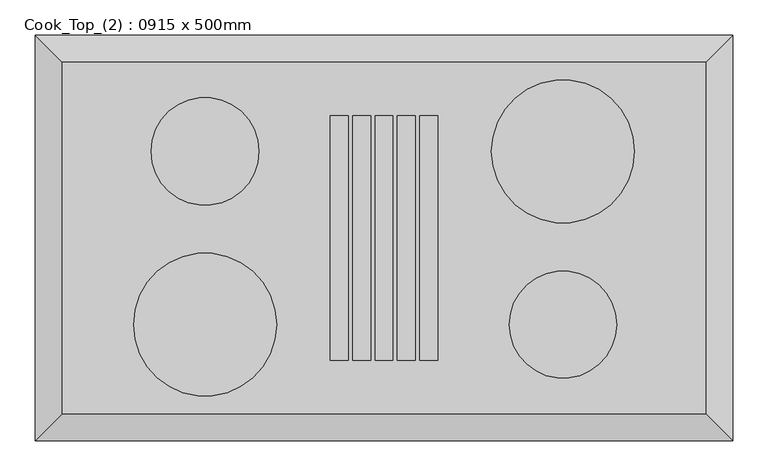
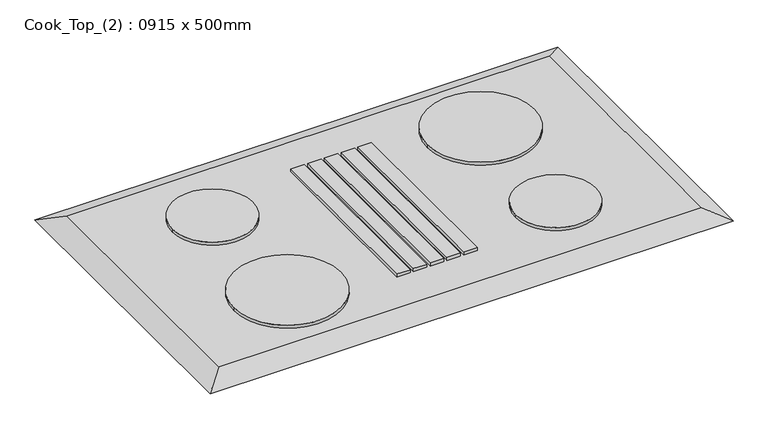
"""IFC4 building model written with IfcOpenShell, lengths in millimetres: proxy geometry, Cook_Top_(2) : 0915 x 500mm."""

from ifc_helpers import new_model, si_unit, point, frame, frame_2d, origin, place, context, project, spatial, polyline, circle_curve, trimmed, segment, composite_curve, outline, extrude, faceted_brep, source, transform, mapped, element, save


def cook_top_2_0915_x_500mm_892363c5(model_context):
    return source(origin(), model_context, "Body", "SolidModel", [
        faceted_brep([(457.5, 250.0, 918.0), (-457.5, 250.0, 918.0), (-457.5, -250.0, 918.0), (457.5, -250.0, 918.0), (495.6, 288.1, 900.0), (495.6, -288.1, 900.0), (-495.6, -288.1, 900.0), (-495.6, 288.1, 900.0)], [[[0, 1, 2, 3]], [[4, 5, 6, 7]], [[4, 7, 1, 0]], [[7, 6, 2, 1]], [[6, 5, 3, 2]], [[5, 4, 0, 3]]]),
        extrude(outline(composite_curve([segment(trimmed(circle_curve(frame_2d((-254.3, 123.0)), 76.5869489), [point((-177.7130511, 123.0))], [point((-330.8869489, 123.0))], False, "CARTESIAN"), True, "CONTINUOUS"), segment(trimmed(circle_curve(frame_2d((-254.3, 123.0)), 76.5869489), [point((-330.8869489, 123.0))], [point((-177.7130511, 123.0))], False, "CARTESIAN"), True, "CONTINUOUS")], self_intersect=False)), frame((0.0, 0.0, 918.0), z_axis=(0.0, 0.0, 1.0), x_axis=(1.0, 0.0, 0.0)), (0.0, 0.0, 1.0), 6.35),
        extrude(outline(composite_curve([segment(trimmed(circle_curve(frame_2d((254.3, 123.0)), 101.6), [point((355.9, 123.0))], [point((152.7, 123.0))], False, "CARTESIAN"), True, "CONTINUOUS"), segment(trimmed(circle_curve(frame_2d((254.3, 123.0)), 101.6), [point((152.7, 123.0))], [point((355.9, 123.0))], False, "CARTESIAN"), True, "CONTINUOUS")], self_intersect=False)), frame((0.0, 0.0, 918.0), z_axis=(0.0, 0.0, 1.0), x_axis=(1.0, 0.0, 0.0)), (0.0, 0.0, 1.0), 6.35),
        extrude(outline(composite_curve([segment(trimmed(circle_curve(frame_2d((254.3, -123.0)), 76.2), [point((330.5, -123.0))], [point((178.1, -123.0))], False, "CARTESIAN"), True, "CONTINUOUS"), segment(trimmed(circle_curve(frame_2d((254.3, -123.0)), 76.2), [point((178.1, -123.0))], [point((330.5, -123.0))], False, "CARTESIAN"), True, "CONTINUOUS")], self_intersect=False)), frame((0.0, 0.0, 918.0), z_axis=(0.0, 0.0, 1.0), x_axis=(1.0, 0.0, 0.0)), (0.0, 0.0, 1.0), 6.35),
        extrude(outline(polyline([(-50.8, 173.8), (-50.8, -173.8), (-76.2, -173.8), (-76.2, 173.8), (-50.8, 173.8)])), frame((0.0, 0.0, 918.0), z_axis=(0.0, 0.0, 1.0), x_axis=(1.0, 0.0, 0.0)), (0.0, 0.0, 1.0), 6.35),
        extrude(outline(polyline([(-19.05, 173.8), (-19.05, -173.8), (-44.45, -173.8), (-44.45, 173.8), (-19.05, 173.8)])), frame((0.0, 0.0, 918.0), z_axis=(0.0, 0.0, 1.0), x_axis=(1.0, 0.0, 0.0)), (0.0, 0.0, 1.0), 6.35),
        extrude(outline(polyline([(12.7, 173.8), (12.7, -173.8), (-12.7, -173.8), (-12.7, 173.8), (12.7, 173.8)])), frame((0.0, 0.0, 918.0), z_axis=(0.0, 0.0, 1.0), x_axis=(1.0, 0.0, 0.0)), (0.0, 0.0, 1.0), 6.35),
        extrude(outline(polyline([(44.45, 173.8), (44.45, -173.8), (19.05, -173.8), (19.05, 173.8), (44.45, 173.8)])), frame((0.0, 0.0, 918.0), z_axis=(0.0, 0.0, 1.0), x_axis=(1.0, 0.0, 0.0)), (0.0, 0.0, 1.0), 6.35),
        extrude(outline(polyline([(76.2, 173.8), (76.2, -173.8), (50.8, -173.8), (50.8, 173.8), (76.2, 173.8)])), frame((0.0, 0.0, 918.0), z_axis=(0.0, 0.0, 1.0), x_axis=(1.0, 0.0, 0.0)), (0.0, 0.0, 1.0), 6.35),
        extrude(outline(composite_curve([segment(trimmed(circle_curve(frame_2d((-254.3, -123.0)), 101.6), [point((-152.7, -123.0))], [point((-355.9, -123.0))], False, "CARTESIAN"), True, "CONTINUOUS"), segment(trimmed(circle_curve(frame_2d((-254.3, -123.0)), 101.6), [point((-355.9, -123.0))], [point((-152.7, -123.0))], False, "CARTESIAN"), True, "CONTINUOUS")], self_intersect=False)), frame((0.0, 0.0, 918.0), z_axis=(0.0, 0.0, 1.0), x_axis=(1.0, 0.0, 0.0)), (0.0, 0.0, 1.0), 6.35),
    ])


if __name__ == "__main__":
    model = new_model("IFC4")
    model_context = context("Model", 3, world=origin())
    ifc_project = project(units=[si_unit("LENGTHUNIT", "METRE", prefix="MILLI")], contexts=[model_context])
    site = spatial("IfcSite", under=ifc_project)
    building = spatial("IfcBuilding", under=site)
    placement = place(None, origin())
    cook_top_2_0915_x_500mm_shape = cook_top_2_0915_x_500mm_892363c5(model_context)
    element("IfcBuildingElementProxy", 1, Name="Cook_Top_(2) : 0915 x 500mm", ObjectType="Cook_Top_(2) : 0915 x 500mm", at=placement, inside=building, context=model_context, shape_type="MappedRepresentation", body=[
        mapped(cook_top_2_0915_x_500mm_shape, transform((0.0, 0.0, 0.0), x_axis=(1.0, 0.0, 0.0), y_axis=(0.0, 1.0, 0.0), z_axis=(0.0, 0.0, 1.0))),
    ])
    save(model, "model.ifc")

# Revit data of these elements
# Type "Cook_Top_(2) : 0915 x 500mm"
#   Keynote = "N"
#   Depth = 500 mm
#   Width = 915 mm
#   Material Burner = Metal - Chrome
#   Material Cooktop = Metal - Steel, Polished
#   Default Elevation = 0
# Element 1 (IfcBuildingElementProxy, "Cook_Top_(2) : 0915 x 500mm")
#   Materials on its faces: "Metal - Chrome", "Metal - Steel, Polished"
# Materials
#   "Metal - Chrome": colour RGB 201 201 201, transparency 0
#   "Metal - Steel, Polished": colour RGB 247 247 247, transparency 0
